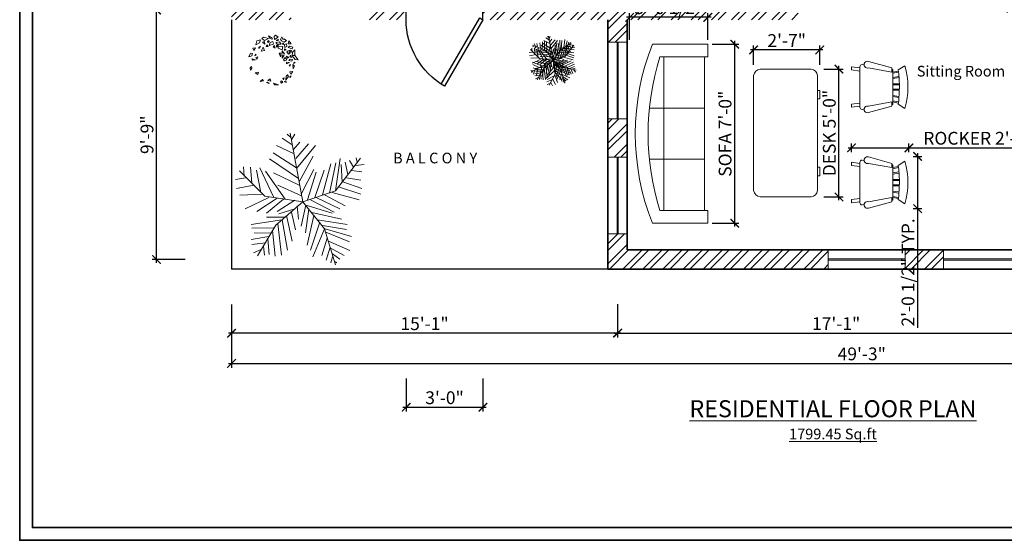
# Model space of a CAD drawing. Units: inches. Extents: x 163 to 947, y 159 to 804.
# Tile 1 of 5: x 163 to 625, y 159 to 403. Entities that reach past the tile are written whole.
import ezdxf

# ---------------------------------------------------------------- set-up
doc = ezdxf.new("R2010")
doc.units = ezdxf.units.IN
for name, color, linetype, lineweight in [('A-ANNO-TEXT', 7, 'Continuous', 18), ('A-ANNO-TTLB', 7, 'Continuous', 35), ('A-AREA-IDEN', 7, 'Continuous', 18), ('A-FLOR-OTLN', 7, 'Continuous', 25), ('Dimensions', 7, 'Continuous', 18), ('Doors', 160, 'Continuous', 25), ('Furniture', 40, 'Continuous', 18), ('Greenary  Plants', 100, 'Continuous', 13), ('Wall Hatch', 214, 'Continuous', 13), ('Walls', 222, 'Continuous', 35), ('Windows', 132, 'Continuous', 18)]:
    doc.layers.add(name, color=color, linetype=linetype, lineweight=lineweight)
doc.styles.get("Standard").update_dxf_attribs({"font": 'arial.ttf'})
doc.dimstyles.new('ISO-25', dxfattribs={"dimtxt": 6, "dimasz": 4, "dimexe": 2, "dimexo": 2, "dimtad": 1, "dimdec": 1, "dimlunit": 3, "dimtxsty": 'Standard', "dimblk": 'ARCHTICK', "dimcen": 0, "dimdle": 1.5, "dimadec": 0, "dimazin": 0, "dimtfac": 1, "dimtdec": 1, "dimtmove": 0, "dimatfit": 3, "dimfxl": 13.5, "dimfxlon": 1, "dimarcsym": 0})

# ---------------------------------------------------------------- blocks, each defined once
blk = doc.blocks.new('_ArchTick')
at = {"color": 0, "linetype": 'ByBlock', "const_width": 0.15}
blk.add_lwpolyline([(-0.5, -0.5), (0.5, 0.5)], dxfattribs=at)
blk = doc.blocks.new('*D12')
at = {"layer": 'Dimensions', "color": 0, "lineweight": -2, "transparency": 16777216}
for p, q in [((262.64, 269.19), (262.64, 253.69)), ((443.62, 269.19), (443.62, 253.69)), ((445.12, 255.69), (261.14, 255.69))]:
    blk.add_line(p, q, dxfattribs=at)
at = {"layer": 'Dimensions', "color": 0, "lineweight": -2, "transparency": 16777216, "xscale": 4, "yscale": 4, "zscale": 4, "rotation": 180}
blk.add_blockref('_ArchTick', (262.64, 255.69), dxfattribs=at)
at = {"layer": 'Dimensions', "color": 0, "lineweight": -2, "transparency": 16777216, "xscale": 4, "yscale": 4, "zscale": 4}
blk.add_blockref('_ArchTick', (443.62, 255.69), dxfattribs=at)
at = {"layer": 'Dimensions', "color": 0, "transparency": 16777216, "insert": (353.13, 259.38), "char_height": 6, "attachment_point": 5}
blk.add_mtext('15\'-1"', dxfattribs=at)
blk = doc.blocks.new('*D13')
at = {"layer": 'Dimensions', "color": 0, "lineweight": -2, "transparency": 16777216}
for p, q in [((443.62, 269.28), (443.62, 253.78)), ((648.62, 269.28), (648.62, 253.78)), ((442.12, 255.78), (650.12, 255.78))]:
    blk.add_line(p, q, dxfattribs=at)
at = {"layer": 'Dimensions', "color": 0, "lineweight": -2, "transparency": 16777216, "xscale": 4, "yscale": 4, "zscale": 4, "rotation": 180}
blk.add_blockref('_ArchTick', (443.62, 255.78), dxfattribs=at)
at = {"layer": 'Dimensions', "color": 0, "lineweight": -2, "transparency": 16777216, "xscale": 4, "yscale": 4, "zscale": 4}
blk.add_blockref('_ArchTick', (648.62, 255.78), dxfattribs=at)
at = {"layer": 'Dimensions', "color": 0, "transparency": 16777216, "insert": (546.12, 259.41), "char_height": 6, "attachment_point": 5}
blk.add_mtext('17\'-1"', dxfattribs=at)
blk = doc.blocks.new('*D15')
at = {"layer": 'Dimensions', "color": 0, "lineweight": -2, "transparency": 16777216}
for p, q in [((240.95, 407.28), (225.45, 407.28)), ((227.45, 288.78), (227.45, 408.78)), ((240.95, 290.28), (225.45, 290.28))]:
    blk.add_line(p, q, dxfattribs=at)
at = {"layer": 'Dimensions', "color": 0, "lineweight": -2, "transparency": 16777216, "xscale": 4, "yscale": 4, "zscale": 4}
for p, rotation in [((227.45, 407.28), 90), ((227.45, 290.28), 270)]:
    blk.add_blockref('_ArchTick', p, dxfattribs=dict(at, rotation=rotation))
at = {"layer": 'Dimensions', "color": 0, "transparency": 16777216, "insert": (223.76, 348.78), "char_height": 6, "attachment_point": 5, "rotation": 90}
blk.add_mtext('9\'-9"', dxfattribs=at)
blk = doc.blocks.new('*U22')
for p, q in [((0, 0), (0, 6)), ((36, 0), (36, 6))]:
    blk.add_line(p, q)
blk.add_lwpolyline([(0, 0), (18, -31.18), (19.52, -30.3), (1.52, 0.88)], close=True)
blk.add_arc((0, 0), 36, 300, 0)
blk = doc.blocks.new('Sofa - Roundback 7 ft.')
for p, q in [((-12.00002, -32.4421), (-12.00003, -6.5971)), ((11.99997, -32.4421), (11.99998, -6.5971)), ((-36.000027, -34), (-36.000027, -11.4696)), ((-35.999844, -13.3819), (35.9998, -13.3819)), ((35.99998, -34), (35.99998, -11.4696)), ((-36.000027, -32.4421), (35.99998, -32.4421))]:
    blk.add_line(p, q)
for points in [[(-36.000027, -34), (-42.000027, -34), (-42.000027, -8)], [(41.99998, -8), (41.99998, -34), (35.99998, -34)]]:
    blk.add_lwpolyline(points)
for centre, radius, start, end in [((0, -114.25), 114.25, 68.43141, 111.5686), ((-0.00001, -127.1968), 121.1968, 72.72033, 107.2797)]:
    blk.add_arc(centre, radius, start, end)
blk = doc.blocks.new('Desk - 30 x 60 in.')
for p, q in [((-26.999995, 0), (26.999995, 0)), ((-29.999995, -27), (-29.999995, -3)), ((29.999995, -3), (29.999995, -27)), ((26.999995, -30), (-26.999995, -30)), ((-20.000005, -30), (-20.000005, -31)), ((-20.000005, -31), (-16.000005, -31)), ((-16.000005, -31), (-16.000005, -30)), ((15.999995, -31), (15.999995, -30)), ((19.999995, -31), (15.999995, -31)), ((19.999995, -30), (19.999995, -31))]:
    blk.add_line(p, q)
for centre, start, end in [((-26.499995, -3.5), 98.1301, 171.8699), ((26.499995, -3.5), 8.130102, 81.8699), ((-26.499995, -26.5), 188.1301, 261.8699), ((26.499995, -26.5), 278.1301, 351.8699)]:
    blk.add_arc(centre, 3.535534, start, end)
blk = doc.blocks.new('Chair - Rocking')
for p, q in [((-8, -4.5), (-10, -1.5)), ((-7.5, -4.5), (-7, -7)), ((-6.5, -7), (-7.02225, -4.43)), ((-4.5, -7), (-4.96674, -4.19951)), ((-4, -7), (-4.40532, -4.16272)), ((-1.5, -4.05012), (-1.5, -7)), ((-1, -7), (-1, -4.05012)), ((1, -7), (1, -4.04655)), ((1.5, -4.05012), (1.5, -7)), ((4, -7), (4.40187, -4.18694)), ((4.5, -7), (4.96761, -4.19437)), ((6.5, -7), (7, -4.4057)), ((7.5, -4.5), (7, -7)), ((8, -4.5), (10, -1.5)), ((-9, -7.5), (-12, -18.49999)), ((-7, -7.5), (-9, -7.5)), ((-9, -18.49999), (-7, -7.5)), ((-8.23428, -6.99939), (-8.3093, -7.47958)), ((-8.23041, -7), (8.23915, -7)), ((7, -7.5), (9, -7.5)), ((9, -18.49999), (7, -7.5)), ((8.31071, -7.48854), (8.23449, -7.00073)), ((9, -7.5), (12, -18.49999)), ((-10.36644, -20.64523), (-10.5, -21.49999)), ((-9, -22.49999), (-9.5, -26.49999)), ((0, -22.49999), (-9.5, -22.49999)), ((-8, -26.49999), (-7.5, -22.49999)), ((0, -22.49999), (9.5, -22.49999)), ((8, -26.49999), (7.5, -22.49999)), ((9, -22.49999), (9.5, -26.49999)), ((10.5, -21.49999), (10.3575, -20.58798)), ((-9.5, -26.49999), (-8, -26.49999)), ((9.5, -26.49999), (8, -26.49999))]:
    blk.add_line(p, q)
for centre, radius, start, end in [((0, -34.08333), 34.08333, 72.93847, 107.0615), ((0, -68.25004), 64.25, 93.92211, 97.15267), ((0, -68.25004), 64.25, 82.84733, 93.92211), ((-10.5, -18.99999), 1.58114, 161.5651, 18.43495), ((-9.5, -21.49999), 1, 180, 270), ((10.5, -18.99999), 1.58114, 161.5651, 18.43495), ((9.5, -21.49999), 1, 270, 0)]:
    blk.add_arc(centre, radius, start, end)
blk = doc.blocks.new('*U54')
for p, q in [((-7.288, 39.707), (-21.778, 46.673)), ((-8.737, 47.138), (-17.069, 52.711)), ((-10.186, 53.64), (-13.084, 55.962)), ((0, 0), (-10.5, 57)), ((-9.099, 51.782), (-6.563, 55.962)), ((-7.65, 43.423), (-2.578, 49.46)), ((-5.839, 35.992), (4.667, 48.067)), ((-5.114, 27.632), (10.463, 46.673)), ((-31.5, 4.5), (-52.5, 25.5)), ((-48.585, 21.131), (-49.309, 29.026)), ((-43.513, 28.561), (-42.427, 15.558)), ((-38.442, 26.239), (-34.819, 7.663)), ((-35.544, 28.097), (-24.314, 3.947)), ((-14.533, 2.09), (-30.834, 25.31)), ((-3.665, 19.273), (-27.574, 35.527)), ((-5.114, 28.097), (-24.676, 40.636)), ((-24.314, 23.917), (-2.941, 13.7)), ((-2.941, 16.486), (8.652, 37.85)), ((-1.129, 6.734), (9.014, 26.704)), ((3.942, 1.625), (11.187, 24.381)), ((10.101, 3.483), (17.708, 26.239)), ((16.259, 5.805), (23.142, 31.348)), ((22.055, 7.198), (27.489, 32.277)), ((27, 9), (48, 36)), ((27.127, 9.056), (31.112, 35.992)), ((31.836, 30.883), (32.561, 16.486)), ((35.096, 32.741), (37.27, 22.524)), ((38.719, 34.134), (41.979, 28.561)), ((40.53, 25.775), (48.862, 24.846)), ((43.791, 29.954), (51.036, 30.883)), ((44.153, 36.456), (45.239, 32.741)), ((-47.498, 19.737), (-55.83, 18.344)), ((-40.615, 13.7), (-55.105, 10.913)), ((-33.37, 6.269), (-52.207, 5.34)), ((-28.299, 3.483), (-47.86, -5.805)), ((-21.416, 3.018), (-38.079, -8.128)), ((0, 0), (-31.5, 4.5)), ((-15.982, 2.09), (-30.11, -9.521)), ((0, 0), (-22.5, -19.5)), ((-6.563, 1.161), (-21.416, -8.128)), ((-20.691, 13.7), (-1.129, 4.876)), ((0, 0), (27, 9)), ((0, 0), (18, -22.5)), ((6.478, 1.625), (26.04, -8.592)), ((11.187, 3.483), (30.749, -5.805)), ((18.07, 5.805), (35.096, -3.483)), ((24.229, 7.663), (46.688, 1.625)), ((29.662, 12.307), (48.137, 6.269)), ((33.285, 16.486), (48.862, 10.913)), ((36.183, 19.737), (48.137, 17.88)), ((-17.431, -15.094), (-42.789, -18.809)), ((-24.314, -21.596), (-42.427, -22.06)), ((-22.5, -19.5), (-37.5, -45)), ((-15.257, -12.772), (-30.11, -12.772)), ((-20.691, -18.345), (-17.793, -44.352)), ((-6.563, -5.805), (-19.967, -9.985)), ((-17.069, -15.094), (-12.721, -40.172)), ((-13.446, -11.378), (-8.737, -32.741)), ((-9.461, -8.592), (-6.201, -23.453)), ((-4.752, -3.483), (-3.665, -14.629)), ((2.493, -3.019), (-1.491, -20.202)), ((1.769, -2.555), (24.229, -9.521)), ((5.029, -6.27), (2.131, -25.775)), ((9.014, -11.378), (3.58, -35.992)), ((14.085, -16.951), (6.478, -40.172)), ((7.565, -9.056), (32.198, -14.629)), ((18.07, -22.524), (8.289, -45.745)), ((12.274, -15.094), (36.907, -18.809)), ((16.259, -19.738), (36.183, -22.989)), ((18, -22.5), (27, -52.5)), ((18.433, -22.524), (40.53, -29.026)), ((-28.299, -29.026), (-42.789, -31.348)), ((-30.834, -34.135), (-42.427, -35.528)), ((-34.457, -39.708), (-40.978, -42.494)), ((-26.849, -26.24), (-40.253, -25.775)), ((-32.646, -36.921), (-31.921, -44.352)), ((-29.023, -30.884), (-27.936, -43.887)), ((-25.038, -23.918), (-22.865, -45.281)), ((20.244, -30.419), (15.897, -44.816)), ((19.157, -25.311), (38.719, -33.206)), ((22.78, -37.85), (19.519, -48.532)), ((21.331, -32.741), (39.081, -40.636)), ((22.78, -38.314), (34.372, -44.816)), ((24.591, -45.745), (23.142, -50.854)), ((24.591, -43.423), (30.749, -47.603)), ((26.764, -49.925), (28.213, -50.854))]:
    blk.add_line(p, q)
blk = doc.blocks.new('*U56')
for points in [[(-147, 248), (-191, 235), (-203, 191), (-159, 215)], [(-113, 281), (-131, 263), (-101, 241), (-53, 263)], [(-49, 241), (-63, 228), (-58, 217), (-46, 230)], [(-51, 296), (-41, 270), (-13, 257), (-5, 270), (-20, 278)], [(31, 305), (14, 287), (19, 254), (64, 281)], [(66, 252), (47, 248), (42, 235), (59, 239)], [(105, 283), (91, 254), (102, 235), (133, 221), (160, 239), (129, 259), (117, 254)], [(189, 237), (181, 202), (217, 202)], [(-207, 153), (-238, 151), (-229, 120)], [(-147, 173), (-169, 158), (-166, 144)], [(-116, 162), (-138, 114), (-99, 122)], [(-123, 219), (-97, 199), (-102, 228)], [(-73, 191), (-80, 169), (-58, 171)], [(1, 230), (-34, 217), (-44, 182), (7, 197)], [(19, 182), (2, 164), (28, 151)], [(35, 217), (79, 224), (97, 199), (49, 197)], [(43, 160), (43, 180), (67, 191), (54, 175)], [(64, 173), (64, 149), (112, 131), (117, 171)], [(117, 210), (115, 197), (126, 193), (126, 210)], [(139, 140), (138, 122), (157, 129)], [(163, 202), (139, 195), (141, 158), (165, 169)], [(206, 127), (181, 118), (165, 105), (187, 79), (206, 90), (194, 98)], [(199, 173), (182, 158), (229, 140), (237, 162)], [(222, 120), (208, 116), (213, 98), (218, 103)], [(261, 131), (234, 103), (229, 59), (266, 13), (299, 10), (263, 63), (237, 61), (261, 72)], [(-287, 46), (-250, 59), (-245, 87), (-265, 90)], [(-209, 10), (-239, 8), (-250, 21)], [(-209, 79), (-215, 59), (-200, 65)], [(-178, 46), (-202, 39), (-190, 13)], [(90, 48), (73, 90), (97, 90)], [(112, 116), (109, 94), (139, 83)], [(109, 70), (134, 68), (112, 32)], [(148, 39), (127, 10), (139, -1), (165, 10)], [(191, 43), (175, 32), (158, 54)], [(206, 19), (191, 4), (227, -7), (232, 13)], [(208, 65), (201, 52), (220, 39)], [(-255, -69), (-270, -84), (-265, -113), (-251, -89)], [(198, -20), (163, -38), (163, -18)], [(211, -45), (203, -64), (193, -53)], [(237, -45), (242, -95), (258, -64)], [(256, -16), (247, -34), (266, -23)], [(-210, -146), (-173, -135), (-178, -165)], [(-123, -225), (-113, -240), (-152, -249)], [(-59, -234), (-32, -216), (-25, -242)], [(134, -203), (117, -207), (127, -227)], [(155, -227), (157, -183), (175, -170), (184, -187)], [(205, -205), (218, -181), (201, -192)], [(237, -130), (215, -159), (203, -132)], [(-65, -256), (-77, -260), (-46, -271)], [(6, -269), (21, -286), (66, -289)], [(103, -240), (90, -253), (103, -269), (117, -251)], [(153, -240), (138, -253), (157, -258)]]:
    blk.add_lwpolyline(points, close=True)
blk = doc.blocks.new('*U57')
for p, q in [((-221.9198, 1197.3052), (-433.5526, 1338.8594)), ((-258.7244, 1362.456), (-332.3336, 1421.4348)), ((0, 0), (-266.7, 1447.8)), ((-231.1146, 1315.2628), (-166.7002, 1421.4348)), ((-194.31, 1102.9442), (-65.4812, 1256.284)), ((-185.1152, 1008.5578), (-553.1612, 1185.4942)), ((-148.3106, 914.1968), (118.5418, 1220.9018)), ((-129.8956, 701.8528), (265.7602, 1185.4942)), ((-93.091, 489.5342), (-700.3796, 902.3858)), ((-129.8956, 713.6638), (-626.7704, 1032.1544)), ((-74.7014, 418.7444), (219.7608, 961.39)), ((685.8, 228.6), (1219.2, 914.4)), ((689.0258, 230.0224), (790.2448, 914.1968)), ((891.4384, 831.6214), (946.658, 572.1096)), ((983.4626, 867.0036), (1066.2666, 725.4494)), ((1121.4862, 925.9824), (1149.0706, 831.6214)), ((-800.1, 114.3), (-1333.5, 647.7)), ((-1234.059, 536.7274), (-1252.4486, 737.2604)), ((-1105.2302, 725.4494), (-1077.6458, 395.1732)), ((-976.4268, 666.4706), (-884.4026, 194.6402)), ((-902.8176, 713.6638), (-617.5756, 100.2538)), ((-369.1382, 53.086), (-783.1836, 642.874)), ((-28.6766, 171.0436), (228.9556, 678.2816)), ((256.5654, 88.4682), (449.7832, 666.4706)), ((412.9786, 147.447), (587.8068, 796.2392)), ((560.197, 182.8292), (698.2206, 819.8358)), ((808.6344, 784.4282), (827.0494, 418.7444)), ((1029.462, 654.685), (1241.0948, 631.0884)), ((1112.2914, 760.8316), (1296.3144, 784.4282)), ((-1206.4492, 501.3198), (-1418.082, 465.9376)), ((-617.5756, 607.4918), (-74.7014, 347.98)), ((100.1268, 41.275), (284.1498, 619.2774)), ((845.439, 418.7444), (1241.0948, 277.1902)), ((919.0482, 501.3198), (1222.6798, 454.152)), ((-1031.621, 347.98), (-1399.667, 277.1902)), ((-525.5514, 347.98), (-28.6766, 123.8504)), ((0, 0), (685.8, 228.6)), ((753.4148, 312.5978), (1222.6798, 159.2326)), ((-847.598, 159.2326), (-1326.0578, 135.636)), ((-718.7946, 88.4682), (-1215.644, -147.447)), ((-543.9664, 76.6572), (-967.2066, -206.4512)), ((0, 0), (-800.1, 114.3)), ((-405.9428, 53.086), (-764.794, -241.8334)), ((0, 0), (-571.5, -495.3)), ((-166.7002, 29.4894), (-543.9664, -206.4512)), ((0, 0), (457.2, -571.5)), ((164.5412, 41.275), (661.416, -218.2368)), ((284.1498, 88.4682), (781.0246, -147.447)), ((458.978, 147.447), (891.4384, -88.4682)), ((615.4166, 194.6402), (1185.8752, 41.275)), ((-166.7002, -147.447), (-507.1618, -253.619)), ((-120.7008, -88.4682), (-93.091, -371.5766)), ((63.3222, -76.6826), (-37.8714, -513.1308)), ((44.9326, -64.897), (615.4166, -241.8334)), ((127.7366, -159.258), (54.1274, -654.685)), ((-442.7474, -383.3876), (-1086.8406, -477.7486)), ((-387.5278, -324.4088), (-764.794, -324.4088)), ((-433.5526, -383.3876), (-323.1134, -1020.3688)), ((-341.5284, -289.0012), (-221.9198, -831.6214)), ((-240.3094, -218.2368), (-157.5054, -595.7062)), ((228.9556, -289.0012), (90.932, -914.1968)), ((192.151, -230.0224), (817.8292, -371.5766)), ((311.7596, -383.3876), (937.4378, -477.7486)), ((-617.5756, -548.5384), (-1077.6458, -560.324)), ((-571.5, -495.3), (-952.5, -1143)), ((-635.9652, -607.5172), (-580.771, -1150.1374)), ((-525.5514, -465.963), (-451.9422, -1126.5408)), ((357.759, -430.5554), (164.5412, -1020.3688)), ((458.978, -572.1096), (210.5406, -1161.923)), ((412.9786, -501.3452), (919.0482, -583.9206)), ((457.2, -571.5), (685.8, -1333.5)), ((468.1982, -572.1096), (1029.462, -737.2604)), ((-718.7946, -737.2604), (-1086.8406, -796.2392)), ((-681.9646, -666.496), (-1022.4262, -654.685)), ((-737.1842, -784.4536), (-709.5744, -1114.7298)), ((514.1976, -772.6426), (403.7838, -1138.3264)), ((486.5878, -642.8994), (983.4626, -843.4324)), ((-783.1836, -867.029), (-1077.6458, -902.4112)), ((-875.2078, -1008.5832), (-1040.8412, -1079.3476)), ((-829.2084, -937.7934), (-810.7934, -1126.5408)), ((578.612, -961.39), (495.7826, -1232.7128)), ((541.8074, -831.6214), (992.6574, -1032.1544)), ((578.612, -973.1756), (873.0488, -1138.3264)), ((624.6114, -1161.923), (587.8068, -1291.6916)), ((624.6114, -1102.9442), (781.0246, -1209.1162)), ((679.8056, -1268.095), (716.6102, -1291.6916))]:
    blk.add_line(p, q)
blk = doc.blocks.new('*D58')
at = {"layer": 'Dimensions', "color": 0, "lineweight": -2, "transparency": 16777216}
for p, q in [((262.64, 255.02), (262.64, 239.52)), ((853.62, 255.02), (853.62, 239.52)), ((261.14, 241.52), (855.12, 241.52))]:
    blk.add_line(p, q, dxfattribs=at)
at = {"layer": 'Dimensions', "color": 0, "lineweight": -2, "transparency": 16777216, "xscale": 4, "yscale": 4, "zscale": 4, "rotation": 180}
blk.add_blockref('_ArchTick', (262.64, 241.52), dxfattribs=at)
at = {"layer": 'Dimensions', "color": 0, "lineweight": -2, "transparency": 16777216, "xscale": 4, "yscale": 4, "zscale": 4}
blk.add_blockref('_ArchTick', (853.62, 241.52), dxfattribs=at)
at = {"layer": 'Dimensions', "color": 0, "transparency": 16777216, "insert": (558.13, 245.21), "char_height": 6, "attachment_point": 5}
blk.add_mtext('49\'-3"', dxfattribs=at)
blk = doc.blocks.new('WIN-36IN')
for p, q in [((0, 9.03), (0, 0)), ((0, 4.76), (35.98, 4.76)), ((35.98, 9.03), (35.98, 0)), ((0, 4.26), (35.98, 4.26))]:
    blk.add_line(p, q)
blk = doc.blocks.new('*D70')
at = {"layer": 'Dimensions', "color": 0, "lineweight": -2, "transparency": 16777216}
for p, q in [((551.77, 342.64), (580.27, 342.64)), ((553.27, 340.59), (553.27, 344.64)), ((580.27, 340.59), (580.27, 344.64)), ((580.27, 342.64), (659.97, 342.64))]:
    blk.add_line(p, q, dxfattribs=at)
at = {"layer": 'Dimensions', "color": 0, "lineweight": -2, "transparency": 16777216, "xscale": 4, "yscale": 4, "zscale": 4, "rotation": 180}
blk.add_blockref('_ArchTick', (553.27, 342.64), dxfattribs=at)
at = {"layer": 'Dimensions', "color": 0, "lineweight": -2, "transparency": 16777216, "xscale": 4, "yscale": 4, "zscale": 4}
blk.add_blockref('_ArchTick', (580.27, 342.64), dxfattribs=at)
at = {"layer": 'Dimensions', "color": 0, "transparency": 16777216, "insert": (622.12, 346.37), "char_height": 6, "attachment_point": 5}
blk.add_mtext('ROCKER 2\'-3" TYP.', dxfattribs=at)
blk = doc.blocks.new('*D71')
at = {"layer": 'Dimensions', "color": 0, "lineweight": -2, "transparency": 16777216}
for p, q in [((582.27, 338.59), (586.32, 338.59)), ((584.32, 340.09), (584.32, 314.15)), ((582.27, 314.15), (586.32, 314.15)), ((584.32, 314.15), (584.32, 258.25))]:
    blk.add_line(p, q, dxfattribs=at)
at = {"layer": 'Dimensions', "color": 0, "lineweight": -2, "transparency": 16777216, "xscale": 4, "yscale": 4, "zscale": 4}
for p, rotation in [((584.32, 338.59), 90), ((584.32, 314.15), 270)]:
    blk.add_blockref('_ArchTick', p, dxfattribs=dict(at, rotation=rotation))
at = {"layer": 'Dimensions', "color": 0, "transparency": 16777216, "insert": (580.59, 284.2), "char_height": 6, "attachment_point": 5, "rotation": 90}
blk.add_mtext('2\'-0 1/2" TYP.', dxfattribs=at)
blk = doc.blocks.new('*D78')
at = {"layer": 'Dimensions', "color": 0, "lineweight": -2, "transparency": 16777216}
for p, q in [((498.55, 305.77), (498.55, 392.77)), ((487.95, 391.27), (500.55, 391.27)), ((487.95, 307.27), (500.55, 307.27))]:
    blk.add_line(p, q, dxfattribs=at)
at = {"layer": 'Dimensions', "color": 0, "lineweight": -2, "transparency": 16777216, "xscale": 4, "yscale": 4, "zscale": 4}
for p, rotation in [((498.55, 391.27), 90), ((498.55, 307.27), 270)]:
    blk.add_blockref('_ArchTick', p, dxfattribs=dict(at, rotation=rotation))
at = {"layer": 'Dimensions', "color": 0, "transparency": 16777216, "insert": (494.82, 349.27), "char_height": 6, "attachment_point": 5, "rotation": 90}
blk.add_mtext('SOFA 7\'-0"', dxfattribs=at)
blk = doc.blocks.new('*D79')
at = {"layer": 'Dimensions', "color": 0, "lineweight": -2, "transparency": 16777216}
for p, q in [((487.45, 403.87), (447.78, 403.87)), ((449.28, 393.27), (449.28, 405.87)), ((485.95, 393.27), (485.95, 405.87))]:
    blk.add_line(p, q, dxfattribs=at)
at = {"layer": 'Dimensions', "color": 0, "lineweight": -2, "transparency": 16777216, "xscale": 4, "yscale": 4, "zscale": 4, "rotation": 180}
blk.add_blockref('_ArchTick', (449.28, 403.87), dxfattribs=at)
at = {"layer": 'Dimensions', "color": 0, "lineweight": -2, "transparency": 16777216, "xscale": 4, "yscale": 4, "zscale": 4}
blk.add_blockref('_ArchTick', (485.95, 403.87), dxfattribs=at)
at = {"layer": 'Dimensions', "color": 0, "transparency": 16777216, "insert": (467.61, 407.6), "char_height": 6, "attachment_point": 5}
blk.add_mtext('3\'-0 1/2"', dxfattribs=at)
blk = doc.blocks.new('*D84')
at = {"layer": 'Dimensions', "color": 0, "lineweight": -2, "transparency": 16777216}
for p, q in [((540.42, 379.59), (549.42, 379.59)), ((547.42, 318.09), (547.42, 381.09)), ((540.42, 319.59), (549.42, 319.59))]:
    blk.add_line(p, q, dxfattribs=at)
at = {"layer": 'Dimensions', "color": 0, "lineweight": -2, "transparency": 16777216, "xscale": 4, "yscale": 4, "zscale": 4}
for p, rotation in [((547.42, 379.59), 90), ((547.42, 319.59), 270)]:
    blk.add_blockref('_ArchTick', p, dxfattribs=dict(at, rotation=rotation))
at = {"layer": 'Dimensions', "color": 0, "transparency": 16777216, "insert": (543.69, 349.59), "char_height": 6, "attachment_point": 5, "rotation": 90}
blk.add_mtext('DESK 5\'-0"', dxfattribs=at)
blk = doc.blocks.new('*D85')
at = {"layer": 'Dimensions', "color": 0, "lineweight": -2, "transparency": 16777216}
for p, q in [((539.92, 388.59), (505.92, 388.59)), ((507.42, 381.59), (507.42, 390.59)), ((538.42, 381.59), (538.42, 390.59))]:
    blk.add_line(p, q, dxfattribs=at)
at = {"layer": 'Dimensions', "color": 0, "lineweight": -2, "transparency": 16777216, "xscale": 4, "yscale": 4, "zscale": 4, "rotation": 180}
blk.add_blockref('_ArchTick', (507.42, 388.59), dxfattribs=at)
at = {"layer": 'Dimensions', "color": 0, "lineweight": -2, "transparency": 16777216, "xscale": 4, "yscale": 4, "zscale": 4}
blk.add_blockref('_ArchTick', (538.42, 388.59), dxfattribs=at)
at = {"layer": 'Dimensions', "color": 0, "transparency": 16777216, "insert": (522.92, 392.23), "char_height": 6, "attachment_point": 5}
blk.add_mtext('2\'-7"', dxfattribs=at)
blk = doc.blocks.new('*D97')
at = {"layer": 'Dimensions', "color": 0, "lineweight": -2, "transparency": 16777216}
for p, q in [((344.51, 234.46), (344.51, 218.96)), ((380.49, 234.46), (380.49, 218.96)), ((343.01, 220.96), (381.99, 220.96))]:
    blk.add_line(p, q, dxfattribs=at)
at = {"layer": 'Dimensions', "color": 0, "lineweight": -2, "transparency": 16777216, "xscale": 4, "yscale": 4, "zscale": 4, "rotation": 180}
blk.add_blockref('_ArchTick', (344.51, 220.96), dxfattribs=at)
at = {"layer": 'Dimensions', "color": 0, "lineweight": -2, "transparency": 16777216, "xscale": 4, "yscale": 4, "zscale": 4}
blk.add_blockref('_ArchTick', (380.49, 220.96), dxfattribs=at)
at = {"layer": 'Dimensions', "color": 0, "transparency": 16777216, "insert": (362.5, 224.65), "char_height": 6, "attachment_point": 5}
blk.add_mtext('3\'-0"', dxfattribs=at)

msp = doc.modelspace()

# ---------------------------------------------------------------- hatches: boundary and pattern name
at = {"layer": 'Wall Hatch'}
h = msp.add_hatch(dxfattribs=at)
h.set_pattern_fill('ANSI32', color=256, scale=0.7)
h.paths.add_polyline_path([(271.66, 713.71), (308.91, 713.71), (308.91, 722.73), (262.64, 722.73), (262.64, 565.31), (271.66, 565.31), (271.66, 583.27), (310.31, 583.27), (310.31, 587.28), (271.66, 587.28)])
h.paths.add_polyline_path([(357.32, 713.71), (400.68, 713.71), (400.68, 722.73), (344.89, 722.73), (344.89, 713.71), (352.3, 713.71), (352.3, 587.28), (340.31, 587.28), (340.31, 583.27), (387.9, 583.27), (387.9, 580.28), (391.92, 580.28), (391.92, 583.27), (411.3, 583.27), (411.3, 587.28), (357.32, 587.28)])
h.paths.add_polyline_path([(454.65, 722.73), (436.66, 722.73), (436.66, 713.71), (444.3, 713.71), (444.3, 587.28), (441.3, 587.28), (441.3, 583.27), (452.32, 583.27), (452.32, 587.28), (449.32, 587.28), (449.32, 713.71), (454.65, 713.71)])
h.paths.add_polyline_path([(546.44, 722.73), (490.63, 722.73), (490.63, 713.71), (537.42, 713.71), (537.42, 587.28), (482.32, 587.28), (482.32, 583.27), (546.44, 583.27), (546.44, 630.27), (552.44, 630.27), (552.44, 639.3), (546.44, 639.3)])
h.paths.add_polyline_path([(271.66, 529.33), (262.64, 529.33), (262.64, 402.77), (290.54, 402.77), (290.54, 411.79), (271.66, 411.79)])
h.paths.add_polyline_path([(344.49, 408.77), (344.51, 411.79), (326.52, 411.79), (326.52, 402.77), (344.49, 402.77)])
h.paths.add_polyline_path([(528.33, 411.79), (510.34, 411.79), (510.34, 521.35), (546.44, 521.35), (546.44, 525.36), (460.92, 525.36), (460.9, 525.35), (460.9, 521.35), (501.32, 521.35), (501.32, 411.79), (390.5, 411.79), (390.5, 521.35), (430.9, 521.35), (430.9, 525.36), (390.5, 525.36), (390.5, 541.96), (386.49, 541.96), (386.49, 411.79), (380.49, 411.79), (380.49, 402.77), (439.11, 402.77), (439.11, 392.26), (448.14, 392.26), (448.14, 402.77), (528.33, 402.77)])
h.paths.add_polyline_path([(448.14, 356.28), (439.11, 356.28), (439.11, 338.29), (448.14, 338.29)])
h.paths.add_polyline_path([(542.45, 294.79), (448.14, 294.79), (448.14, 302.31), (439.11, 302.31), (439.11, 285.77), (542.45, 285.77)])
h.paths.add_polyline_path([(596.42, 294.79), (578.43, 294.79), (578.43, 285.77), (596.42, 285.77)])
h.paths.add_polyline_path([(653.12, 402.77), (659.11, 402.77), (659.11, 408.77), (659.11, 411.79), (626.1, 411.79), (626.1, 402.77), (644.09, 402.77), (644.09, 294.79), (632.4, 294.79), (632.4, 285.77), (653.12, 285.77)])
h.paths.add_polyline_path([(738.49, 630.27), (844.6, 630.27), (844.6, 603.27), (853.62, 603.27), (853.62, 722.73), (663.29, 722.73), (663.29, 677.29), (672.32, 677.29), (672.32, 713.71), (777.6, 713.71), (777.6, 669.29), (783.62, 669.29), (783.62, 713.71), (844.6, 713.71), (844.6, 636.29), (783.62, 636.29), (783.62, 639.29), (777.6, 639.29), (777.6, 636.29), (672.32, 636.29), (672.32, 645.29), (663.29, 645.29), (663.29, 639.3), (582.43, 639.3), (582.43, 630.27), (643.22, 630.27), (643.22, 624.27), (648.23, 624.27), (648.23, 630.27), (732.47, 630.27), (732.47, 547.43), (648.23, 547.43), (648.23, 594.27), (643.22, 594.27), (643.22, 525.36), (625.17, 525.36), (625.17, 517.34), (648.23, 517.34), (648.23, 541.41), (729.47, 541.41), (729.47, 517.34), (738.49, 517.34)])
h.paths.add_polyline_path([(853.62, 567.29), (844.6, 567.29), (844.6, 489.33), (853.62, 489.33)])
h.paths.add_polyline_path([(853.62, 453.35), (844.6, 453.35), (844.6, 411.79), (826.3, 411.79), (826.3, 402.77), (853.62, 402.77)])
h.paths.add_polyline_path([(790.32, 411.79), (772.33, 411.79), (772.33, 402.77), (790.32, 402.77)])
h.paths.add_polyline_path([(736.35, 411.79), (695.11, 411.79), (695.11, 402.77), (736.35, 402.77)])

# ---------------------------------------------------------------- linework, layer by layer
at = {"layer": 'A-ANNO-TTLB'}
for points in [[(163.29, 792.35), (947.45, 792.35), (947.45, 158.54), (163.29, 158.54)], [(169.29, 786.35), (941.45, 786.35), (941.45, 164.54), (169.29, 164.54)]]:
    msp.add_lwpolyline(points, close=True, dxfattribs=at)
at = {"layer": 'A-FLOR-OTLN'}
for p in [(262.64, 402.77), (439.11, 285.77)]:
    msp.add_line(p, (262.64, 285.77), dxfattribs=at)
at = {"layer": 'Walls'}
for p, q in [((439.11, 402.77), (439.11, 285.77)), ((448.14, 402.77), (448.14, 294.79)), ((448.14, 294.79), (644.09, 294.79)), ((439.11, 285.77), (653.12, 285.77))]:
    msp.add_line(p, q, dxfattribs=at)

# ---------------------------------------------------------------- block references
at = {"layer": 'Doors', "xscale": -1}
msp.add_blockref('*U22', (380.49, 402.77), dxfattribs=at)
at = {"layer": 'Furniture'}
for name, p, rotation in [('Sofa - Roundback 7 ft.', (451.95, 349.27), 90), ('Chair - Rocking', (579.77, 371.18), 269.9999849999999), ('Desk - 30 x 60 in.', (507.42, 349.59), 90), ('Chair - Rocking', (579.77, 326.37), 269.9999849999999)]:
    msp.add_blockref(name, p, dxfattribs=dict(at, rotation=rotation))
at = {"layer": 'Greenary  Plants'}
for name, p, xscale, yscale, zscale in [('*U56', (282.02, 383.52), 0.0393700787401575, 0.0393700787401575, 0.0393700787401575), ('*U54', (413.4, 383.61), 0.2010375495604706, 0.2010375495604706, 0.2010375495604706), ('*U57', (296.04, 317.39), 0.0222440134676828, 0.0222440134676828, 0.0222440134676828)]:
    msp.add_blockref(name, p, dxfattribs=dict(at, xscale=xscale, yscale=yscale, zscale=zscale))
at = {"layer": 'Greenary  Plants', "xscale": 0.2010375495604706, "yscale": 0.2010375495604706, "zscale": 0.2010375495604706, "rotation": 106.8221293867638}
msp.add_blockref('*U54', (413.4, 383.61), dxfattribs=at)
at = {"layer": 'Windows', "rotation": 90.00000000000017}
for p in [(448.14, 356.28), (448.14, 302.31)]:
    msp.add_blockref('WIN-36IN', p, dxfattribs=at)
at = {"layer": 'Windows'}
for p in [(542.45, 285.77), (596.42, 285.77)]:
    msp.add_blockref('WIN-36IN', p, dxfattribs=at)

# ---------------------------------------------------------------- texts
at = {"layer": 'A-ANNO-TEXT', "insert": (369.04, 224.26), "char_height": 8, "attachment_point": 1}
msp.add_mtext_dynamic_manual_height_columns('\\pxsm1.5,qc;{\\fTimes New Roman|b1|i0|c0|p18;\\T2.15;\\LRESIDENTIAL\\l \\LFLOOR\\l \\LPLAN\\P\\ps*;\\H0.625x;\\T1.05;1799.45 Sq.ft}', width=351.123, gutter_width=12.5, heights=[0], dxfattribs=at)
at = {"layer": 'A-AREA-IDEN', "char_height": 5, "attachment_point": 1}
for s, width, insert in [('\\pxqc;{\\fTimes New Roman|b0|i0|c0|p18;Sitting Room}', 42.9286, (583.18, 381.11)), ('\\pxqc;{\\fTimes New Roman|b0|i0|c0|p18;B A L C O N Y}', 56.611, (329.78, 340.37))]:
    msp.add_mtext_dynamic_manual_height_columns(s, width=width, gutter_width=12.5, heights=[0], dxfattribs=dict(at, insert=insert))

# ---------------------------------------------------------------- dimensions: what is measured, and where the dimension line sits
at = {"layer": 'Dimensions'}
for base, p1, p2, angle, override, picture, middle in [((449.28, 403.87), (485.95, 391.27), (449.28, 391.27), 180, {"dimdec": 1, "dimlfac": 1, "dimrnd": 0, "dimzin": 1, "dimdsep": 46, "dimlunit": 4, "dimfrac": 2}, '*D79', (467.61, 407.6)), ((227.45, 407.28), (256.15, 290.28), (256.15, 407.28), 90, {"dimclrd": 0, "dimclre": 0, "dimclrt": 0}, '*D15', (223.76, 348.78)), ((507.42, 388.59), (538.42, 379.59), (507.42, 379.59), 180, {"dimdec": 1, "dimlfac": 1, "dimrnd": 0, "dimzin": 1, "dimdsep": 46, "dimlunit": 4, "dimfrac": 2}, '*D85', (522.92, 392.23))]:
    dim = msp.add_linear_dim(base=base, p1=p1, p2=p2, angle=angle, dimstyle='ISO-25', override=override, dxfattribs=at)
    dim.commit()
    dim.dimension.update_dxf_attribs({"geometry": picture, "text_midpoint": middle})
for base, p1, p2, override, picture, middle in [((380.49, 220.96), (344.51, 402.77), (380.49, 402.77), {"dimdec": 1, "dimlfac": 1, "dimrnd": 0, "dimzin": 1, "dimdsep": 46, "dimlunit": 4, "dimfrac": 2}, '*D97', (362.5, 224.65)), ((853.62, 241.52), (262.64, 285.77), (853.62, 285.77), {"dimclrd": 0, "dimclre": 0, "dimclrt": 0}, '*D58', (558.13, 245.21)), ((648.62, 255.78), (443.62, 281.76), (648.62, 281.76), {"dimclrd": 0, "dimclre": 0, "dimclrt": 0}, '*D13', (546.12, 259.41)), ((262.64, 255.69), (443.62, 277.24), (262.64, 277.24), {"dimclrd": 0, "dimclre": 0, "dimclrt": 0}, '*D12', (353.13, 259.38))]:
    dim = msp.add_linear_dim(base=base, p1=p1, p2=p2, dimstyle='ISO-25', override=override, dxfattribs=at)
    dim.commit()
    dim.dimension.update_dxf_attribs({"geometry": picture, "text_midpoint": middle})
for base, p1, p2, angle, text, picture, middle in [((498.55, 391.27), (485.95, 307.27), (485.95, 391.27), 90, 'SOFA <>', '*D78', (494.82, 349.27)), ((547.42, 379.59), (538.42, 319.59), (538.42, 379.59), 90, 'DESK <>', '*D84', (543.69, 349.59)), ((580.27, 342.64), (553.27, 338.59), (580.27, 338.59), 360, 'ROCKER <> TYP.', '*D70', (622.12, 346.37)), ((584.32, 314.15), (580.27, 338.59), (580.27, 314.15), 270, '<> TYP.', '*D71', (580.59, 284.2))]:
    dim = msp.add_linear_dim(base=base, p1=p1, p2=p2, angle=angle, text=text, dimstyle='ISO-25', override={"dimdec": 1, "dimlfac": 1, "dimrnd": 0, "dimzin": 1, "dimdsep": 46, "dimlunit": 4, "dimfrac": 2}, dxfattribs=at)
    dim.commit()
    dim.dimension.update_dxf_attribs({"geometry": picture, "text_midpoint": middle})

doc.saveas('drawing.dxf')
